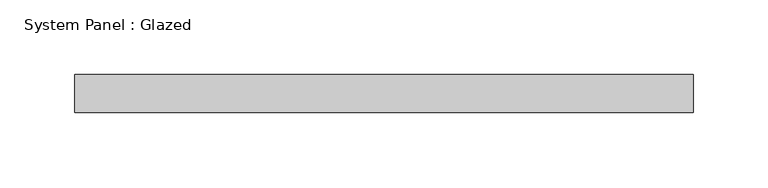
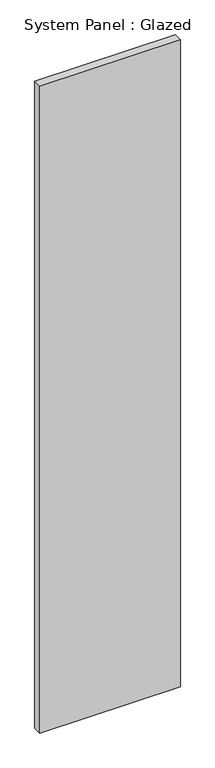
"""IFC4 building model written with IfcOpenShell, lengths in millimetres: plate geometry, System Panel : Glazed."""

from ifc_helpers import new_model, si_unit, origin, origin_with_axes, place, context, project, spatial, polyline, outline, extrude, source, transform, mapped, element, save


def system_panel_glazed_74c9e8f4(model_context):
    return source(origin(), model_context, "Body", "SweptSolid", [
        extrude(outline(polyline([(206.375, 19.05), (-206.375, 19.05), (-206.375, 44.45), (206.375, 44.45), (206.375, 19.05)])), origin_with_axes(), (0.0, 0.0, 1.0), 2006.6),
    ])


if __name__ == "__main__":
    model = new_model("IFC4")
    model_context = context("Model", 3, world=origin())
    ifc_project = project(units=[si_unit("LENGTHUNIT", "METRE", prefix="MILLI")], contexts=[model_context])
    site = spatial("IfcSite", under=ifc_project)
    building = spatial("IfcBuilding", under=site)
    placement = place(None, origin())
    system_panel_glazed_shape = system_panel_glazed_74c9e8f4(model_context)
    element("IfcPlate", 1, ObjectType="System Panel : Glazed", at=placement, inside=building, context=model_context, shape_type="MappedRepresentation", body=[
        mapped(system_panel_glazed_shape, transform((0.0, 0.0, 0.0), x_axis=(1.0, 0.0, 0.0), y_axis=(0.0, 1.0, 0.0), z_axis=(0.0, 0.0, 1.0))),
    ])
    save(model, "model.ifc")

# Revit data of these elements
# Type "System Panel : Glazed"
#   Construction Type Id = "GSP4R"
#   Analytic Construction = "1/8 in Pilkington single glazing"
#   Visual Light Transmittance = 0.9
#   Solar Heat Gain Coefficient = 0.86
#   Heat Transfer Coefficient (U) = 1.18115 BTU/(h·ft²·°F)
#   Define Thermal Properties by = 1
# Element 1 (IfcPlate, "System Panel : Glazed")
#   Materials on its faces: "Glass"
# Materials
#   "Glass": class "Glass", colour RGB 0 128 192, transparency 0.75, Description = "Soda Lime Glass", Cost = 0
